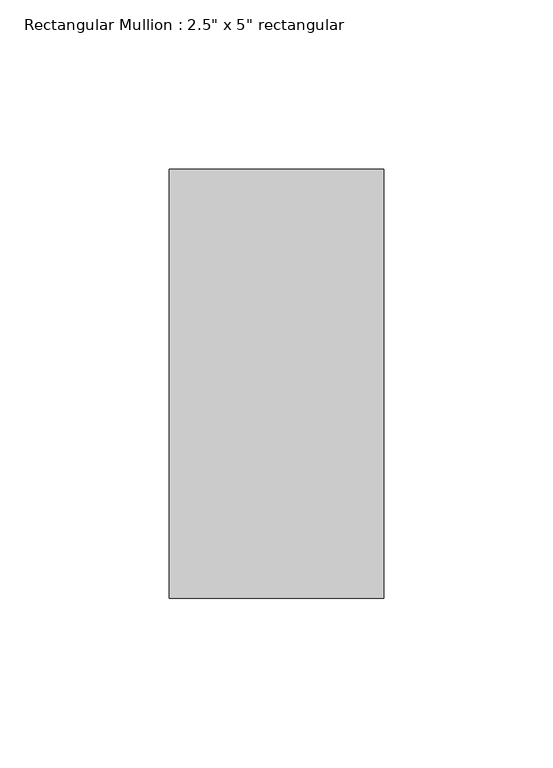
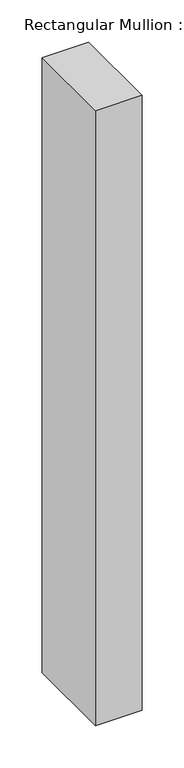
"""IFC4 building model written with IfcOpenShell, lengths in millimetres: member geometry."""

from ifc_helpers import new_model, si_unit, frame, origin, place, context, project, spatial, polyline, outline, extrude, source, transform, mapped, element, save


def member_26863f11(model_context):
    return source(origin(), model_context, "Body", "SweptSolid", [
        extrude(outline(polyline([(0.0, 63.5), (0.0, -63.5), (-63.5, -63.5), (-63.5, 63.5), (0.0, 63.5)])), frame((0.0, 0.0, -889.0), z_axis=(0.0, 0.0, 1.0), x_axis=(1.0, 0.0, 0.0)), (0.0, 0.0, 1.0), 889.0),
    ])


if __name__ == "__main__":
    model = new_model("IFC4")
    model_context = context("Model", 3, world=origin())
    ifc_project = project(units=[si_unit("LENGTHUNIT", "METRE", prefix="MILLI")], contexts=[model_context])
    site = spatial("IfcSite", under=ifc_project)
    building = spatial("IfcBuilding", under=site)
    placement = place(None, origin())
    member_shape = member_26863f11(model_context)
    element("IfcMember", 1, ObjectType="Rectangular Mullion : 2.5\" x 5\" rectangular", at=placement, inside=building, context=model_context, shape_type="MappedRepresentation", body=[
        mapped(member_shape, transform((0.0, 0.0, 0.0), x_axis=(1.0, 0.0, 0.0), y_axis=(0.0, 1.0, 0.0), z_axis=(0.0, 0.0, 1.0))),
    ])
    save(model, "model.ifc")

# Revit data of these elements
# Type "Rectangular Mullion : 2.5\" x 5\" rectangular"
#   built-in parameter 1007304 = 0.416667 (stored number, unit not read)
#   built-in parameter 1007301 = 0.104167 (stored number, unit not read)
#   built-in parameter 1007300 = 0.104167 (stored number, unit not read)
# Element 1 (IfcMember, "Rectangular Mullion : 2.5\" x 5\" rectangular")
#   Materials on its faces: "Aluminum"
# Materials
#   "Aluminum": class "Metal", colour RGB 247 247 247, transparency 0, Description = "Aluminum 6061", Cost = 0
